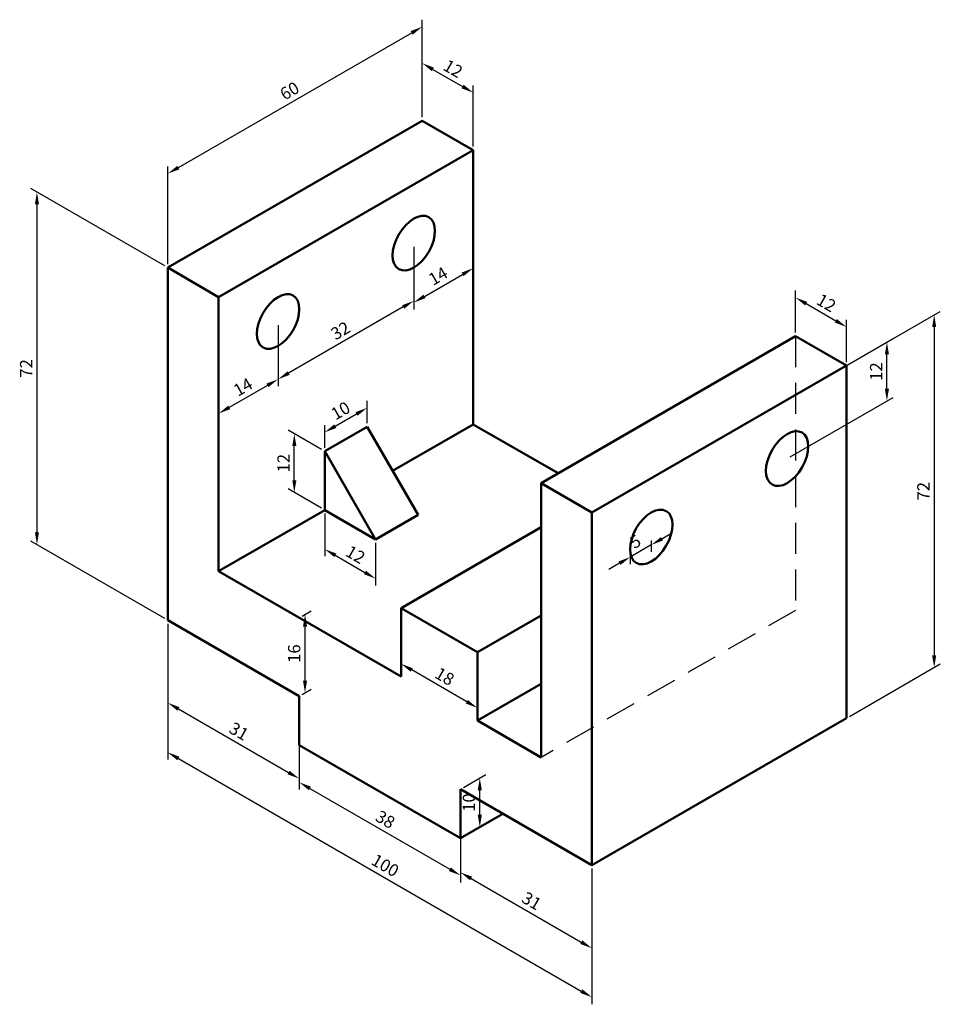
# Model space of a CAD drawing. Units: millimetres. Extents: x 126 to 314, y -25 to 176.
import ezdxf

# ---------------------------------------------------------------- set-up
doc = ezdxf.new("R2010")
doc.units = ezdxf.units.MM
doc.linetypes.add('HIDDEN', pattern=[9.525, 6.35, -3.175])
for name, color, linetype, lineweight in [('M-DIMS', 2, 'Continuous', 25), ('M-HIDN', 4, 'HIDDEN', 25), ('M-OUTL', 7, 'Continuous', 50)]:
    doc.layers.add(name, color=color, linetype=linetype, lineweight=lineweight)
doc.styles.get("Standard").update_dxf_attribs({"font": 'arial.ttf'})
doc.dimstyles.new('ISO-25', dxfattribs={"dimtxt": 2.5, "dimasz": 2.5, "dimexe": 1.25, "dimexo": 0.625, "dimtad": 1, "dimtxsty": 'Standard', "dimcen": 2.5, "dimadec": 0, "dimazin": 0, "dimtfac": 1, "dimtmove": 0, "dimatfit": 3, "dimfxl": 1, "dimarcsym": 0})

# ---------------------------------------------------------------- blocks, each defined once
blk = doc.blocks.new('*D1')
at = {"layer": 'Defpoints', "color": 0, "transparency": 16777216}
for p in [(215.96, 18.48), (242.81, 2.98), (242.81, -14)]:
    blk.add_point(p, dxfattribs=at)
at = {"layer": 'M-DIMS', "color": 0, "lineweight": -2, "transparency": 16777216}
for p, q in [((215.96, 17.76), (215.96, 0.06)), ((242.81, 2.26), (242.81, -15.44)), ((218.12, 0.25), (240.64, -12.75))]:
    blk.add_line(p, q, dxfattribs=at)
at = {"layer": 'M-DIMS', "color": 0, "transparency": 16777216}
for points in [[(218.33, 0.62), (217.92, -0.11), (215.96, 1.5)], [(240.85, -12.38), (240.43, -13.11), (242.81, -14)]]:
    blk.add_solid(points, dxfattribs=at)
at = {"layer": 'M-DIMS', "color": 0, "transparency": 16777216, "insert": (230.33, -4.6), "char_height": 2.5, "attachment_point": 5, "rotation": 330}
blk.add_mtext('31', dxfattribs=at)
blk = doc.blocks.new('*D2')
at = {"layer": 'Defpoints', "color": 0, "transparency": 16777216}
for p in [(183.05, 27.48), (215.96, 8.48), (215.96, 0.89)]:
    blk.add_point(p, dxfattribs=at)
at = {"layer": 'M-DIMS', "color": 0, "lineweight": -2, "transparency": 16777216}
for p, q in [((183.05, 26.76), (183.05, 18.45)), ((185.21, 18.64), (213.79, 2.14)), ((215.96, 7.76), (215.96, -0.55))]:
    blk.add_line(p, q, dxfattribs=at)
at = {"layer": 'M-DIMS', "color": 0, "transparency": 16777216}
for points in [[(185.42, 19), (185.01, 18.28), (183.05, 19.89)], [(214, 2.5), (213.59, 1.78), (215.96, 0.89)]]:
    blk.add_solid(points, dxfattribs=at)
at = {"layer": 'M-DIMS', "color": 0, "transparency": 16777216, "insert": (200.46, 12.04), "char_height": 2.5, "attachment_point": 5, "rotation": 330}
blk.add_mtext('38', dxfattribs=at)
blk = doc.blocks.new('*D3')
at = {"layer": 'Defpoints', "color": 0, "transparency": 16777216}
for p in [(156.2, 52.98), (183.05, 37.48), (183.05, 20.63)]:
    blk.add_point(p, dxfattribs=at)
at = {"layer": 'M-DIMS', "color": 0, "lineweight": -2, "transparency": 16777216}
for p, q in [((156.2, 52.26), (156.2, 34.69)), ((183.05, 36.76), (183.05, 19.19)), ((158.37, 34.88), (180.88, 21.88))]:
    blk.add_line(p, q, dxfattribs=at)
at = {"layer": 'M-DIMS', "color": 0, "transparency": 16777216}
for points in [[(158.58, 35.24), (158.16, 34.52), (156.2, 36.13)], [(181.09, 22.24), (180.68, 21.52), (183.05, 20.63)]]:
    blk.add_solid(points, dxfattribs=at)
at = {"layer": 'M-DIMS', "color": 0, "transparency": 16777216, "insert": (170.58, 30.03), "char_height": 2.5, "attachment_point": 5, "rotation": 330}
blk.add_mtext('31', dxfattribs=at)
blk = doc.blocks.new('*D4')
at = {"layer": 'Defpoints', "color": 0, "transparency": 16777216}
for p in [(156.2, 52.98), (242.81, 2.98), (242.81, -23.99)]:
    blk.add_point(p, dxfattribs=at)
at = {"layer": 'M-DIMS', "color": 0, "lineweight": -2, "transparency": 16777216}
for p, q in [((156.2, 52.26), (156.2, 24.56)), ((158.37, 24.76), (240.64, -22.74)), ((242.81, 2.26), (242.81, -25.44))]:
    blk.add_line(p, q, dxfattribs=at)
at = {"layer": 'M-DIMS', "color": 0, "transparency": 16777216}
for points in [[(158.58, 25.12), (158.16, 24.39), (156.2, 26.01)], [(240.85, -22.38), (240.43, -23.11), (242.81, -23.99)]]:
    blk.add_solid(points, dxfattribs=at)
at = {"layer": 'M-DIMS', "color": 0, "transparency": 16777216, "insert": (200.45, 2.65), "char_height": 2.5, "attachment_point": 5, "rotation": 330}
blk.add_mtext('100', dxfattribs=at)
blk = doc.blocks.new('*D5')
at = {"layer": 'Defpoints', "color": 0, "transparency": 16777216}
for p in [(294.77, 104.98), (312.68, 43.33), (294.77, 32.98)]:
    blk.add_point(p, dxfattribs=at)
at = {"layer": 'M-DIMS', "color": 0, "lineweight": -2, "transparency": 16777216}
for p, q in [((295.39, 105.34), (313.93, 116.05)), ((312.68, 112.83), (312.68, 45.83)), ((295.39, 33.34), (313.93, 44.05))]:
    blk.add_line(p, q, dxfattribs=at)
at = {"layer": 'M-DIMS', "color": 0, "transparency": 16777216}
for points in [[(312.26, 112.83), (313.1, 112.83), (312.68, 115.33)], [(312.26, 45.83), (313.1, 45.83), (312.68, 43.33)]]:
    blk.add_solid(points, dxfattribs=at)
at = {"layer": 'M-DIMS', "color": 0, "transparency": 16777216, "insert": (310.8, 79.33), "char_height": 2.5, "attachment_point": 5, "rotation": 90}
blk.add_mtext('72', dxfattribs=at)
blk = doc.blocks.new('*D6')
at = {"layer": 'Defpoints', "color": 0, "transparency": 16777216}
for p in [(303.03, 109.76), (282.64, 97.98), (282.64, 85.98)]:
    blk.add_point(p, dxfattribs=at)
at = {"layer": 'M-DIMS', "color": 0, "lineweight": -2, "transparency": 16777216}
for p, q in [((283.27, 98.34), (304.28, 110.48)), ((303.03, 100.26), (303.03, 107.26)), ((283.27, 86.34), (304.28, 98.48))]:
    blk.add_line(p, q, dxfattribs=at)
at = {"layer": 'M-DIMS', "color": 0, "transparency": 16777216}
for points in [[(302.61, 107.26), (303.45, 107.26), (303.03, 109.76)], [(302.61, 100.26), (303.45, 100.26), (303.03, 97.76)]]:
    blk.add_solid(points, dxfattribs=at)
at = {"layer": 'M-DIMS', "color": 0, "transparency": 16777216, "insert": (301.15, 103.76), "char_height": 2.5, "attachment_point": 5, "rotation": 90}
blk.add_mtext('12', dxfattribs=at)
blk = doc.blocks.new('*D7')
at = {"layer": 'Defpoints', "color": 0, "transparency": 16777216}
for p in [(294.77, 112.88), (284.37, 110.98), (294.77, 104.98)]:
    blk.add_point(p, dxfattribs=at)
at = {"layer": 'M-DIMS', "color": 0, "lineweight": -2, "transparency": 16777216}
for p, q in [((284.37, 111.71), (284.37, 120.33)), ((286.54, 117.63), (292.6, 114.13)), ((294.77, 105.71), (294.77, 114.33))]:
    blk.add_line(p, q, dxfattribs=at)
at = {"layer": 'M-DIMS', "color": 0, "transparency": 16777216}
for points in [[(286.75, 117.99), (286.33, 117.27), (284.37, 118.88)], [(292.81, 114.49), (292.39, 113.77), (294.77, 112.88)]]:
    blk.add_solid(points, dxfattribs=at)
at = {"layer": 'M-DIMS', "color": 0, "transparency": 16777216, "insert": (290.51, 117.51), "char_height": 2.5, "attachment_point": 5, "rotation": 330}
blk.add_mtext('12', dxfattribs=at)
blk = doc.blocks.new('*D8')
at = {"layer": 'Defpoints', "color": 0, "transparency": 16777216}
for p in [(218.56, 160.72), (208.16, 154.98), (218.56, 148.98)]:
    blk.add_point(p, dxfattribs=at)
at = {"layer": 'M-DIMS', "color": 0, "lineweight": -2, "transparency": 16777216}
for p, q in [((208.16, 155.71), (208.16, 168.16)), ((210.33, 165.47), (216.39, 161.97)), ((218.56, 149.71), (218.56, 162.16))]:
    blk.add_line(p, q, dxfattribs=at)
at = {"layer": 'M-DIMS', "color": 0, "transparency": 16777216}
for points in [[(210.54, 165.83), (210.12, 165.1), (208.16, 166.72)], [(216.6, 162.33), (216.18, 161.6), (218.56, 160.72)]]:
    blk.add_solid(points, dxfattribs=at)
at = {"layer": 'M-DIMS', "color": 0, "transparency": 16777216, "insert": (214.3, 165.34), "char_height": 2.5, "attachment_point": 5, "rotation": 330}
blk.add_mtext('12', dxfattribs=at)
blk = doc.blocks.new('*D9')
at = {"layer": 'Defpoints', "color": 0, "transparency": 16777216}
for p in [(218.56, 136.98), (206.43, 129.98), (218.56, 124.86)]:
    blk.add_point(p, dxfattribs=at)
at = {"layer": 'M-DIMS', "color": 0, "lineweight": -2, "transparency": 16777216}
for p, q in [((218.56, 136.26), (218.56, 123.42)), ((206.43, 129.26), (206.43, 116.42)), ((208.6, 119.11), (216.39, 123.61))]:
    blk.add_line(p, q, dxfattribs=at)
at = {"layer": 'M-DIMS', "color": 0, "transparency": 16777216}
for points in [[(216.18, 123.97), (216.6, 123.25), (218.56, 124.86)], [(208.39, 119.47), (208.81, 118.75), (206.43, 117.86)]]:
    blk.add_solid(points, dxfattribs=at)
at = {"layer": 'M-DIMS', "color": 0, "transparency": 16777216, "insert": (211.55, 122.99), "char_height": 2.5, "attachment_point": 5, "rotation": 30}
blk.add_mtext('14', dxfattribs=at)
blk = doc.blocks.new('*D10')
at = {"layer": 'Defpoints', "color": 0, "transparency": 16777216}
for p in [(206.43, 129.98), (178.72, 113.98), (178.72, 102.2)]:
    blk.add_point(p, dxfattribs=at)
at = {"layer": 'M-DIMS', "color": 0, "lineweight": -2, "transparency": 16777216}
for p, q in [((206.43, 129.26), (206.43, 116.75)), ((204.27, 116.95), (180.88, 103.45)), ((178.72, 113.26), (178.72, 100.75))]:
    blk.add_line(p, q, dxfattribs=at)
at = {"layer": 'M-DIMS', "color": 0, "transparency": 16777216}
for points in [[(204.06, 117.31), (204.48, 116.59), (206.43, 118.2)], [(180.68, 103.81), (181.09, 103.09), (178.72, 102.2)]]:
    blk.add_solid(points, dxfattribs=at)
at = {"layer": 'M-DIMS', "color": 0, "transparency": 16777216, "insert": (191.62, 111.84), "char_height": 2.5, "attachment_point": 5, "rotation": 30}
blk.add_mtext('32', dxfattribs=at)
blk = doc.blocks.new('*D11')
at = {"layer": 'Defpoints', "color": 0, "transparency": 16777216}
for p in [(178.72, 113.98), (166.6, 106.98), (166.6, 95.2)]:
    blk.add_point(p, dxfattribs=at)
at = {"layer": 'M-DIMS', "color": 0, "lineweight": -2, "transparency": 16777216}
for p, q in [((178.72, 113.26), (178.72, 100.75)), ((166.6, 106.26), (166.6, 93.75)), ((176.55, 100.95), (168.76, 96.45))]:
    blk.add_line(p, q, dxfattribs=at)
at = {"layer": 'M-DIMS', "color": 0, "transparency": 16777216}
for points in [[(176.35, 101.31), (176.76, 100.59), (178.72, 102.2)], [(168.55, 96.81), (168.97, 96.09), (166.6, 95.2)]]:
    blk.add_solid(points, dxfattribs=at)
at = {"layer": 'M-DIMS', "color": 0, "transparency": 16777216, "insert": (171.72, 100.33), "char_height": 2.5, "attachment_point": 5, "rotation": 30}
blk.add_mtext('14', dxfattribs=at)
blk = doc.blocks.new('*D12')
at = {"layer": 'Defpoints', "color": 0, "transparency": 16777216}
for p in [(188.25, 75.48), (198.64, 69.48), (198.64, 61.49)]:
    blk.add_point(p, dxfattribs=at)
at = {"layer": 'M-DIMS', "color": 0, "lineweight": -2, "transparency": 16777216}
for p, q in [((188.25, 74.76), (188.25, 66.05)), ((198.64, 68.76), (198.64, 60.05)), ((190.41, 66.24), (196.47, 62.74))]:
    blk.add_line(p, q, dxfattribs=at)
at = {"layer": 'M-DIMS', "color": 0, "transparency": 16777216}
for points in [[(190.62, 66.6), (190.2, 65.88), (188.25, 67.49)], [(196.68, 63.1), (196.26, 62.38), (198.64, 61.49)]]:
    blk.add_solid(points, dxfattribs=at)
at = {"layer": 'M-DIMS', "color": 0, "transparency": 16777216, "insert": (194.38, 66.12), "char_height": 2.5, "attachment_point": 5, "rotation": 330}
blk.add_mtext('12', dxfattribs=at)
blk = doc.blocks.new('*D13')
at = {"layer": 'Defpoints', "color": 0, "transparency": 16777216}
for p in [(196.91, 96.36), (196.91, 92.48), (188.25, 87.48)]:
    blk.add_point(p, dxfattribs=at)
at = {"layer": 'M-DIMS', "color": 0, "lineweight": -2, "transparency": 16777216}
for p, q in [((196.91, 93.21), (196.91, 97.8)), ((190.41, 92.61), (194.74, 95.11)), ((188.25, 88.21), (188.25, 92.8))]:
    blk.add_line(p, q, dxfattribs=at)
at = {"layer": 'M-DIMS', "color": 0, "transparency": 16777216}
for points in [[(194.53, 95.47), (194.95, 94.75), (196.91, 96.36)], [(190.2, 92.97), (190.62, 92.25), (188.25, 91.36)]]:
    blk.add_solid(points, dxfattribs=at)
at = {"layer": 'M-DIMS', "color": 0, "transparency": 16777216, "insert": (191.63, 95.5), "char_height": 2.5, "attachment_point": 5, "rotation": 30}
blk.add_mtext('10', dxfattribs=at)
blk = doc.blocks.new('*D14')
at = {"layer": 'Defpoints', "color": 0, "transparency": 16777216}
for p in [(182.04, 91.06), (188.25, 87.48), (188.25, 75.48)]:
    blk.add_point(p, dxfattribs=at)
at = {"layer": 'M-DIMS', "color": 0, "lineweight": -2, "transparency": 16777216}
for p, q in [((187.62, 87.84), (180.79, 91.79)), ((182.04, 81.56), (182.04, 88.56)), ((187.62, 75.84), (180.79, 79.79))]:
    blk.add_line(p, q, dxfattribs=at)
at = {"layer": 'M-DIMS', "color": 0, "transparency": 16777216}
for points in [[(181.63, 88.56), (182.46, 88.56), (182.04, 91.06)], [(181.63, 81.56), (182.46, 81.56), (182.04, 79.06)]]:
    blk.add_solid(points, dxfattribs=at)
at = {"layer": 'M-DIMS', "color": 0, "transparency": 16777216, "insert": (180.16, 85.06), "char_height": 2.5, "attachment_point": 5, "rotation": 90}
blk.add_mtext('12', dxfattribs=at)
blk = doc.blocks.new('*D15')
at = {"layer": 'Defpoints', "color": 0, "transparency": 16777216}
for p in [(203.83, 55.48), (219.42, 46.48), (203.83, 44.09)]:
    blk.add_point(p, dxfattribs=at)
at = {"layer": 'M-DIMS', "color": 0, "lineweight": -2, "transparency": 16777216}
for p, q in [((203.83, 54.76), (203.83, 42.65)), ((219.42, 45.76), (219.42, 33.65)), ((217.26, 36.34), (206, 42.84))]:
    blk.add_line(p, q, dxfattribs=at)
at = {"layer": 'M-DIMS', "color": 0, "transparency": 16777216}
for points in [[(206.21, 43.2), (205.79, 42.48), (203.83, 44.09)], [(217.47, 36.7), (217.05, 35.98), (219.42, 35.09)]]:
    blk.add_solid(points, dxfattribs=at)
at = {"layer": 'M-DIMS', "color": 0, "transparency": 16777216, "insert": (212.58, 41.24), "char_height": 2.5, "attachment_point": 5, "rotation": 330}
blk.add_mtext('18', dxfattribs=at)
blk = doc.blocks.new('*D16')
at = {"layer": 'Defpoints', "color": 0, "transparency": 16777216}
for p in [(183.05, 53.48), (184.23, 54.17), (183.05, 37.48)]:
    blk.add_point(p, dxfattribs=at)
at = {"layer": 'M-DIMS', "color": 0, "lineweight": -2, "transparency": 16777216}
for p, q in [((183.67, 53.84), (185.48, 54.89)), ((184.23, 40.67), (184.23, 51.67)), ((183.67, 37.84), (185.48, 38.89))]:
    blk.add_line(p, q, dxfattribs=at)
at = {"layer": 'M-DIMS', "color": 0, "transparency": 16777216}
for points in [[(183.81, 51.67), (184.65, 51.67), (184.23, 54.17)], [(183.81, 40.67), (184.65, 40.67), (184.23, 38.17)]]:
    blk.add_solid(points, dxfattribs=at)
at = {"layer": 'M-DIMS', "color": 0, "transparency": 16777216, "insert": (182.33, 46.17), "char_height": 2.5, "attachment_point": 5, "rotation": 90}
blk.add_mtext('16', dxfattribs=at)
blk = doc.blocks.new('*D17')
at = {"layer": 'Defpoints', "color": 0, "transparency": 16777216}
for p in [(156.2, 124.98), (129.49, 68.41), (156.2, 52.98)]:
    blk.add_point(p, dxfattribs=at)
at = {"layer": 'M-DIMS', "color": 0, "lineweight": -2, "transparency": 16777216}
for p, q in [((155.58, 125.34), (128.24, 141.13)), ((129.49, 137.91), (129.49, 70.91)), ((155.58, 53.34), (128.24, 69.13))]:
    blk.add_line(p, q, dxfattribs=at)
at = {"layer": 'M-DIMS', "color": 0, "transparency": 16777216}
for points in [[(129.08, 137.91), (129.91, 137.91), (129.49, 140.41)], [(129.08, 70.91), (129.91, 70.91), (129.49, 68.41)]]:
    blk.add_solid(points, dxfattribs=at)
at = {"layer": 'M-DIMS', "color": 0, "transparency": 16777216, "insert": (127.61, 104.41), "char_height": 2.5, "attachment_point": 5, "rotation": 90}
blk.add_mtext('72', dxfattribs=at)
blk = doc.blocks.new('*D18')
at = {"layer": 'Defpoints', "color": 0, "transparency": 16777216}
for p in [(208.16, 174.17), (208.16, 154.98), (156.2, 124.98)]:
    blk.add_point(p, dxfattribs=at)
at = {"layer": 'M-DIMS', "color": 0, "lineweight": -2, "transparency": 16777216}
for p, q in [((208.16, 155.71), (208.16, 175.61)), ((158.37, 145.42), (206, 172.92)), ((156.2, 125.71), (156.2, 145.61))]:
    blk.add_line(p, q, dxfattribs=at)
at = {"layer": 'M-DIMS', "color": 0, "transparency": 16777216}
for points in [[(205.79, 173.28), (206.21, 172.56), (208.16, 174.17)], [(158.16, 145.78), (158.58, 145.06), (156.2, 144.17)]]:
    blk.add_solid(points, dxfattribs=at)
at = {"layer": 'M-DIMS', "color": 0, "transparency": 16777216, "insert": (181.23, 160.81), "char_height": 2.5, "attachment_point": 5, "rotation": 30}
blk.add_mtext('60', dxfattribs=at)
blk = doc.blocks.new('*D19')
at = {"layer": 'Defpoints', "color": 0, "transparency": 16777216}
for p in [(219.91, 20.76), (215.96, 18.48), (215.96, 8.48)]:
    blk.add_point(p, dxfattribs=at)
at = {"layer": 'M-DIMS', "color": 0, "lineweight": -2, "transparency": 16777216}
for p, q in [((216.58, 18.84), (221.16, 21.49)), ((219.91, 13.26), (219.91, 18.26)), ((216.58, 8.84), (221.16, 11.49))]:
    blk.add_line(p, q, dxfattribs=at)
at = {"layer": 'M-DIMS', "color": 0, "transparency": 16777216}
for points in [[(219.49, 18.26), (220.33, 18.26), (219.91, 20.76)], [(219.49, 13.26), (220.33, 13.26), (219.91, 10.76)]]:
    blk.add_solid(points, dxfattribs=at)
at = {"layer": 'M-DIMS', "color": 0, "transparency": 16777216, "insert": (218.01, 15.76), "char_height": 2.5, "attachment_point": 5, "rotation": 90}
blk.add_mtext('10', dxfattribs=at)
blk = doc.blocks.new('*D20')
at = {"layer": 'Defpoints', "color": 0, "transparency": 16777216}
for p in [(254.93, 69.98), (250.6, 67.48), (250.6, 65.87)]:
    blk.add_point(p, dxfattribs=at)
at = {"layer": 'M-DIMS', "color": 0, "lineweight": -2, "transparency": 16777216}
for p, q in [((257.09, 69.62), (259.26, 70.87)), ((254.93, 68.37), (250.6, 65.87)), ((254.93, 69.26), (254.93, 66.92)), ((250.6, 66.76), (250.6, 64.42)), ((248.43, 64.62), (246.27, 63.37))]:
    blk.add_line(p, q, dxfattribs=at)
at = {"layer": 'M-DIMS', "color": 0, "transparency": 16777216}
for points in [[(256.89, 69.98), (257.3, 69.26), (254.93, 68.37)], [(248.23, 64.98), (248.64, 64.26), (250.6, 65.87)]]:
    blk.add_solid(points, dxfattribs=at)
at = {"layer": 'M-DIMS', "color": 0, "transparency": 16777216, "insert": (251.82, 68.76), "char_height": 2.5, "attachment_point": 5, "rotation": 30}
blk.add_mtext('5', dxfattribs=at)

msp = doc.modelspace()

# ---------------------------------------------------------------- linework, layer by layer
at = {"layer": 'M-HIDN'}
for p, q in [((284.375, 110.984), (284.375, 54.984)), ((284.375, 54.984), (232.413, 24.984)), ((284.375, 54.984), (262.724, 42.484))]:
    msp.add_line(p, q, dxfattribs=at)
at = {"layer": 'M-OUTL'}
for p, q in [((156.203, 124.984), (208.164, 154.984)), ((208.164, 154.984), (218.557, 148.984)), ((218.557, 148.984), (166.595, 118.984)), ((218.557, 148.984), (218.557, 92.984)), ((166.595, 118.984), (156.203, 124.984)), ((156.203, 124.984), (156.203, 52.984)), ((166.595, 62.984), (166.595, 118.984)), ((232.413, 80.984), (284.375, 110.984)), ((284.375, 110.984), (294.767, 104.984)), ((242.805, 74.984), (294.767, 104.984)), ((294.767, 104.984), (294.767, 32.984)), ((188.246, 87.484), (196.906, 92.484)), ((207.298, 74.484), (196.906, 92.484)), ((202.102, 83.484), (218.557, 92.984)), ((218.557, 92.984), (235.877, 82.984)), ((188.246, 75.484), (188.246, 87.484)), ((198.638, 69.484), (188.246, 87.484)), ((242.805, 74.984), (232.413, 80.984)), ((232.413, 80.984), (232.413, 24.984)), ((166.595, 62.984), (188.246, 75.484)), ((188.246, 75.484), (198.638, 69.484)), ((198.638, 69.484), (207.298, 74.484)), ((242.805, 2.984), (242.805, 74.984)), ((203.834, 55.484), (232.413, 71.984)), ((203.834, 41.484), (166.595, 62.984)), ((219.423, 46.484), (203.834, 55.484)), ((203.834, 55.484), (203.834, 41.484)), ((156.203, 52.984), (183.05, 37.484)), ((219.423, 46.484), (232.413, 53.984)), ((219.423, 46.484), (219.423, 32.484)), ((219.423, 32.484), (232.413, 39.984)), ((183.05, 37.484), (183.05, 27.484)), ((232.413, 24.984), (219.423, 32.484)), ((294.767, 32.984), (242.805, 2.984)), ((183.05, 27.484), (215.959, 8.484)), ((215.959, 8.484), (215.959, 18.484)), ((215.959, 18.484), (242.805, 2.984)), ((215.959, 8.484), (224.619, 13.484))]:
    msp.add_line(p, q, dxfattribs=at)
for centre in [(206.432, 129.984), (178.719, 113.984), (282.643, 85.984), (254.93, 69.984)]:
    msp.add_ellipse(centre, major_axis=(-3.062, -5.303), ratio=0.5773503, dxfattribs=at)

# ---------------------------------------------------------------- dimensions: what is measured, and where the dimension line sits
at = {"layer": 'M-DIMS'}
for p1, p2, distance, picture, middle in [((156.203, 124.984), (208.164, 154.984), 16.613, '*D18', (181.233, 160.814)), ((208.164, 154.984), (218.557, 148.984), 10.16, '*D8', (214.301, 165.344)), ((206.432, 129.984), (218.557, 136.984), -10.499, '*D9', (211.554, 122.989)), ((206.432, 129.984), (178.719, 113.984), 10.208, '*D10', (191.625, 111.845)), ((284.375, 110.984), (294.767, 104.984), 6.842, '*D7', (290.511, 117.512)), ((178.719, 113.984), (166.595, 106.984), 10.208, '*D11', (171.717, 100.325)), ((188.246, 87.484), (196.906, 92.484), 3.355, '*D13', (191.625, 95.504)), ((188.246, 75.484), (198.638, 69.484), -6.922, '*D12', (194.382, 66.119)), ((254.93, 69.984), (250.6, 67.484), 1.4, '*D20', (251.816, 68.759)), ((219.423, 46.484), (203.834, 55.484), 9.864, '*D15', (212.579, 41.24)), ((156.203, 52.984), (183.05, 37.484), -14.593, '*D3', (170.577, 30.031)), ((156.203, 52.984), (242.805, 2.984), -23.364, '*D4', (200.455, 2.652)), ((183.05, 27.484), (215.959, 8.484), -6.577, '*D2', (200.455, 12.037)), ((215.959, 18.484), (242.805, 2.984), -14.705, '*D1', (230.333, -4.598))]:
    dim = msp.add_aligned_dim(p1=p1, p2=p2, distance=distance, dimstyle='ISO-25', override={"dimclrd": 0, "dimclre": 0, "dimclrt": 0}, dxfattribs=at)
    dim.commit()
    dim.dimension.update_dxf_attribs({"geometry": picture, "text_midpoint": middle})
for base, p1, p2, picture, middle in [((129.492, 68.405), (156.203, 124.984), (156.203, 52.984), '*D17', (127.612, 104.405)), ((312.681, 43.327), (294.767, 104.984), (294.767, 32.984), '*D5', (310.801, 79.327)), ((303.031, 109.755), (282.643, 85.984), (282.643, 97.984), '*D6', (301.151, 103.755)), ((182.044, 91.064), (188.246, 75.484), (188.246, 87.484), '*D14', (180.164, 85.064)), ((184.23, 54.166), (183.05, 37.484), (183.05, 53.484), '*D16', (182.329, 46.166)), ((219.909, 20.764), (215.959, 8.484), (215.959, 18.484), '*D19', (218.007, 15.764))]:
    dim = msp.add_linear_dim(base=base, p1=p1, p2=p2, angle=90, dimstyle='ISO-25', override={"dimclrd": 0, "dimclre": 0, "dimclrt": 0}, dxfattribs=at)
    dim.commit()
    dim.dimension.update_dxf_attribs({"geometry": picture, "text_midpoint": middle})

doc.saveas('drawing.dxf')
